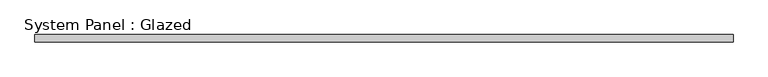
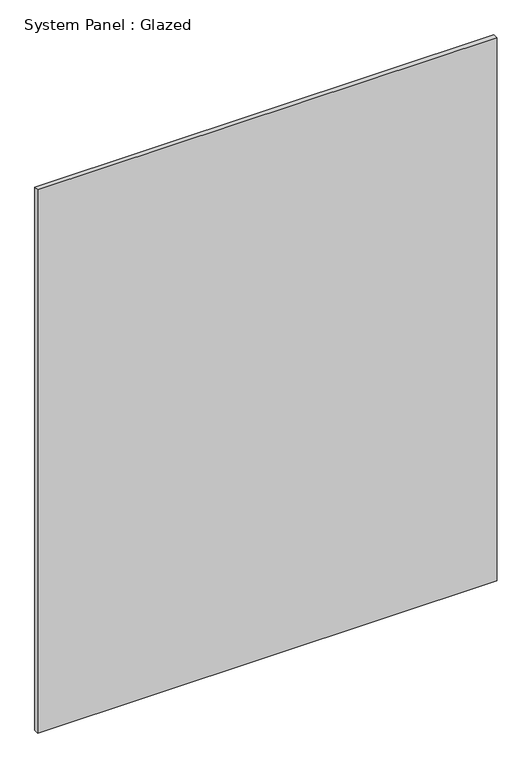
"""IFC4 building model written with IfcOpenShell, lengths in millimetres: plate geometry, System Panel : Glazed."""

from ifc_helpers import new_model, si_unit, origin, origin_with_axes, place, context, project, spatial, polyline, outline, extrude, source, transform, mapped, element, save


def system_panel_glazed_c60cfc80(model_context):
    return source(origin(), model_context, "Body", "SweptSolid", [
        extrude(outline(polyline([(1219.2, 19.05), (-1219.2, 19.05), (-1219.2, 44.45), (1219.2, 44.45), (1219.2, 19.05)])), origin_with_axes(), (0.0, 0.0, 1.0), 3048.0),
    ])


if __name__ == "__main__":
    model = new_model("IFC4")
    model_context = context("Model", 3, world=origin())
    ifc_project = project(units=[si_unit("LENGTHUNIT", "METRE", prefix="MILLI")], contexts=[model_context])
    site = spatial("IfcSite", under=ifc_project)
    building = spatial("IfcBuilding", under=site)
    placement = place(None, origin())
    system_panel_glazed_shape = system_panel_glazed_c60cfc80(model_context)
    element("IfcPlate", 1, ObjectType="System Panel : Glazed", at=placement, inside=building, context=model_context, shape_type="MappedRepresentation", body=[
        mapped(system_panel_glazed_shape, transform((0.0, 0.0, 0.0), x_axis=(1.0, 0.0, 0.0), y_axis=(0.0, 1.0, 0.0), z_axis=(0.0, 0.0, 1.0))),
    ])
    save(model, "model.ifc")

# Revit data of these elements
# Type "System Panel : Glazed"
#   Construction Type Id = "GSP4R"
#   Analytic Construction = "1/8 in Pilkington single glazing"
#   Visual Light Transmittance = 0.9
#   Solar Heat Gain Coefficient = 0.86
#   Heat Transfer Coefficient (U) = 1.18115 BTU/(h·ft²·°F)
# Element 1 (IfcPlate, "System Panel : Glazed")
#   Materials on its faces: "Glass"
# Materials
#   "Glass": class "Glass", colour RGB 0 128 192, transparency 0.75, Description = "Soda Lime Glass", Cost = 0
